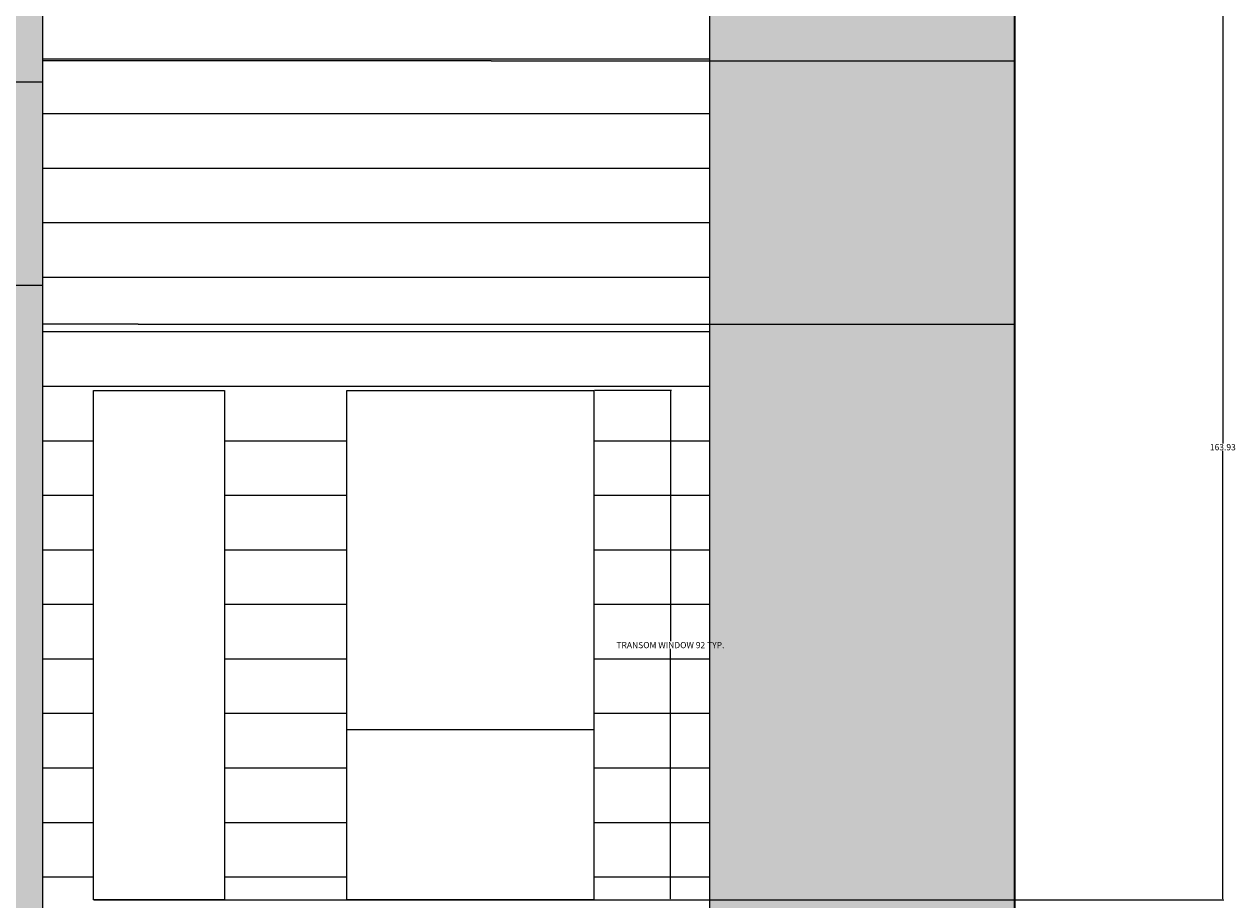
# Model space of a CAD drawing. Units: inches. Extents: x 8 to 634, y 41 to 867.
# Tile 9 of 21: x 415 to 634, y 124 to 283. Entities that reach past the tile are written whole.
import ezdxf

# ---------------------------------------------------------------- set-up
doc = ezdxf.new("R2010")
doc.units = ezdxf.units.IN
doc.header["$MEASUREMENT"] = 0
for name, color, linetype, lineweight in [('A-ANNO-DIMS', 2, 'Continuous', 18), ('A-GLAZ', 4, 'Continuous', 25), ('A-WALL', 7, 'Continuous', 35), ('A-WALL-PANL', 7, 'Continuous', 18), ('A-WALL-PATT', 8, 'Continuous', 9)]:
    doc.layers.add(name, color=color, linetype=linetype, lineweight=lineweight)
doc.styles.get("Standard").update_dxf_attribs({"font": 'arial.ttf'})
doc.dimstyles.get("Standard").update_dxf_attribs({"dimtxt": 1.125, "dimasz": 0.18, "dimexe": 0.18, "dimexo": 0.0625, "dimgap": 0.09, "dimtad": 0, "dimtih": 1, "dimtoh": 1, "dimdec": 4, "dimzin": 0, "dimdsep": 46, "dimlunit": 4, "dimtxsty": 'Standard', "dimcen": 0.09, "dimadec": 0, "dimazin": 0, "dimtfac": 1, "dimtdec": 4, "dimtofl": 0, "dimtmove": 0, "dimatfit": 3, "dimfxl": 1, "dimtolj": 1, "dimtzin": 0, "dimarcsym": 0})

# ---------------------------------------------------------------- blocks, each defined once
blk = doc.blocks.new('WIN-NARROW-FIXED')
blk.add_lwpolyline([(0, 92.26), (23.77, 92.26), (23.77, 0), (0, 0)], close=True)
blk = doc.blocks.new('WIN-WIDE-TRANSOM')
blk.add_line((0, 30.85), (44.78, 30.85))
blk.add_lwpolyline([(0, 92.26), (44.78, 92.26), (44.78, 0), (0, 0)], close=True)
blk = doc.blocks.new('*D9')
at = {"layer": 'A-ANNO-DIMS', "color": 0, "lineweight": -2, "transparency": 16777216}
for p, q in [((518.18, 216.5), (532.13, 216.5)), ((531.95, 216.32), (531.95, 171.04)), ((531.95, 124.41), (531.95, 169.69)), ((518.18, 124.23), (532.13, 124.23))]:
    blk.add_line(p, q, dxfattribs=at)
at = {"layer": 'A-ANNO-DIMS', "color": 0, "transparency": 16777216}
for points in [[(531.92, 216.32), (531.98, 216.32), (531.95, 216.5)], [(531.92, 124.41), (531.98, 124.41), (531.95, 124.23)]]:
    blk.add_solid(points, dxfattribs=at)
at = {"layer": 'Defpoints', "color": 0, "transparency": 16777216}
for p in [(518.11, 216.5), (531.95, 216.5), (518.11, 124.23)]:
    blk.add_point(p, dxfattribs=at)
at = {"layer": 'A-ANNO-DIMS', "color": 0, "transparency": 16777216, "insert": (531.95, 170.36), "char_height": 1.125, "attachment_point": 5}
blk.add_mtext('\\A1;TRANSOM WINDOW 92 TYP.', dxfattribs=at)
blk = doc.blocks.new('*D39')
at = {"layer": 'A-ANNO-DIMS', "color": 0, "lineweight": -2, "transparency": 16777216}
for p, q in [((427.5, 288.17), (632.18, 288.17)), ((632, 287.99), (632, 206.86)), ((632, 124.41), (632, 205.54)), ((427.5, 124.23), (632.18, 124.23))]:
    blk.add_line(p, q, dxfattribs=at)
at = {"layer": 'A-ANNO-DIMS', "color": 0, "transparency": 16777216}
for points in [[(631.97, 287.99), (632.03, 287.99), (632, 288.17)], [(631.97, 124.41), (632.03, 124.41), (632, 124.23)]]:
    blk.add_solid(points, dxfattribs=at)
at = {"layer": 'Defpoints', "color": 0, "transparency": 16777216}
for p in [(427.44, 288.17), (632, 288.17), (427.44, 124.23)]:
    blk.add_point(p, dxfattribs=at)
at = {"layer": 'A-ANNO-DIMS', "color": 0, "transparency": 16777216, "insert": (632, 206.2), "char_height": 1.125, "attachment_point": 5}
blk.add_mtext('\\A1;163.93', dxfattribs=at)

msp = doc.modelspace()

# ---------------------------------------------------------------- hatches: boundary and pattern name
at = {"layer": 'A-WALL-PATT', "transparency": 33554687}
h = msp.add_hatch(dxfattribs=at)
h.set_pattern_fill('ANSI31', color=256, scale=79, angle=135)
h.paths.add_polyline_path([(539.0002, 276.166), (499.4677, 276.166), (418.2881, 276.166), (418.2881, 228.4951), (435.5682, 228.4951), (539.0002, 228.4951)])
h.paths.add_polyline_path([(539.0002, 228.4951), (435.5682, 228.4951), (418.2881, 228.4951), (418.2881, 112.2342), (439.3242, 112.2342), (539.0002, 112.2342)])
h.paths.add_polyline_path([(518.1129, 124.2342), (473.3277, 124.2342), (473.3277, 216.4951), (518.1129, 216.4951)], flags=16)
h.paths.add_polyline_path([(451.2116, 124.2342), (427.4368, 124.2342), (427.4368, 216.4951), (451.2116, 216.4951)], flags=16)
h.paths.add_polyline_path([(539.0002, 112.2342), (439.3242, 112.2342), (418.2881, 112.2342), (418.2881, 91.5417), (539.0002, 91.5417)])
h.paths.add_polyline_path([(539.0002, 392.4268), (427.4368, 392.4268), (418.2881, 392.4268), (418.2881, 391.7598), (418.2881, 276.166), (499.4677, 276.166), (539.0002, 276.166)])
h.paths.add_polyline_path([(518.1129, 288.166), (473.3277, 288.166), (473.3277, 380.4268), (518.1129, 380.4268)], flags=16)
h.paths.add_polyline_path([(451.2116, 288.166), (427.4368, 288.166), (427.4368, 380.4268), (451.2116, 380.4268)], flags=16)
h.paths.add_polyline_path([(539.0002, 451.6305), (427.4368, 452.9097), (418.2881, 452.9097), (418.2881, 392.4268), (427.4368, 392.4268), (539.0002, 392.4268)])
h.paths.add_polyline_path([(539.0002, 569.1705), (427.4368, 569.1705), (418.2881, 569.1705), (418.2881, 452.9097), (427.4368, 452.9097), (539.0002, 451.6305)])
h.paths.add_polyline_path([(473.3277, 557.1705), (518.1129, 557.1705), (518.1129, 464.9097), (473.3277, 464.9097)], flags=16)
h.paths.add_polyline_path([(451.2116, 557.1705), (451.2116, 464.9097), (427.4368, 464.9097), (427.4368, 557.1705)], flags=16)
h.paths.add_polyline_path([(539.0002, 619.6298), (418.2881, 619.6298), (418.2881, 569.1705), (427.4368, 569.1705), (539.0002, 569.1705)])
h.paths.add_polyline_path([(556.7072, 774.3342), (556.7072, 776.8929), (299.7961, 776.8929), (299.7961, 697.6655), (322.56, 697.6655), (322.56, 740.5561), (355.7466, 740.5561), (355.7466, 697.6655), (360.785, 697.6655), (370.3877, 697.6655), (370.3877, 740.5561), (439.201, 740.5561), (439.201, 691.978), (449.4498, 691.978), (449.4498, 740.5561), (498.2535, 740.5561), (498.2535, 691.978), (508.5023, 691.978), (508.5023, 740.5561), (536.3204, 740.5561), (536.3204, 691.978), (539.0002, 691.978), (539.0002, 697.6655), (556.7072, 697.6655)])
h = msp.add_hatch(dxfattribs=at)
h.set_pattern_fill('AR-CONC', color=256, scale=3.2)
h.paths.add_polyline_path([(119.7065, 697.6655), (47.3401, 697.6655), (47.3401, 569.1705), (119.7065, 569.1705)])
h.paths.add_polyline_path([(202.1558, 697.6655), (119.7065, 697.6655), (119.7065, 569.1705), (202.1558, 569.1705)])
h.paths.add_polyline_path([(284.6051, 697.6655), (202.1558, 697.6655), (202.1558, 569.1705), (284.6051, 569.1705)])
h.paths.add_polyline_path([(119.7065, 569.1705), (47.3401, 569.1705), (47.3401, 523.5555), (47.3401, 449.7533), (119.7065, 449.7533)])
h.paths.add_polyline_path([(342.6544, 682.1444), (360.785, 697.6655), (284.6051, 697.6655), (284.6051, 569.1705), (342.6544, 569.1705)])
h.paths.add_polyline_path([(342.6544, 569.1705), (284.6051, 569.1705), (284.6051, 449.7533), (342.6544, 449.7533)])
h.paths.add_polyline_path([(418.2881, 691.978), (418.2881, 697.6655), (360.785, 697.6655), (360.785, 569.1705), (418.2881, 569.1705)])
h.paths.add_polyline_path([(418.2881, 569.1705), (360.785, 569.1705), (360.785, 523.5555), (360.785, 449.7533), (418.2881, 449.7533)])
h.paths.add_polyline_path([(594.3501, 697.6655), (539.0002, 697.6655), (539.0002, 691.978), (539.0002, 569.1705), (594.3501, 569.1705)])
h.paths.add_polyline_path([(594.3501, 523.5555), (594.3501, 569.1705), (539.0002, 569.1705), (539.0002, 451.6305), (594.3501, 451.6305)])
h.paths.add_polyline_path([(594.3501, 451.6305), (539.0002, 451.6305), (539.0002, 391.7598), (594.3501, 391.7598)])
h.paths.add_polyline_path([(594.3501, 391.7598), (539.0002, 391.7598), (539.0002, 276.166), (594.3501, 276.166)])
h.paths.add_polyline_path([(418.2881, 449.7533), (360.785, 449.7533), (360.785, 391.7598), (418.2881, 391.7598)])
h.paths.add_polyline_path([(342.6544, 449.7533), (284.6051, 449.7533), (284.6051, 391.7598), (342.6544, 391.7598)])
h.paths.add_polyline_path([(342.6544, 391.7598), (284.6051, 391.7598), (284.6051, 272.3426), (342.6544, 272.3426)])
h.paths.add_polyline_path([(418.2881, 391.7598), (360.785, 391.7598), (360.785, 272.3426), (418.2881, 272.3426)])
h.paths.add_polyline_path([(418.2881, 272.3426), (360.785, 272.3426), (360.785, 235.5555), (418.2881, 235.5555)])
h.paths.add_polyline_path([(342.6544, 272.3426), (284.6051, 272.3426), (284.6051, 235.5555), (295.0049, 235.5555), (342.6544, 235.5555)])
h.paths.add_polyline_path([(594.3501, 276.166), (539.0002, 276.166), (539.0002, 228.4951), (594.3501, 228.4951)])
h.paths.add_polyline_path([(594.3501, 228.4951), (539.0002, 228.4951), (539.0002, 91.5417), (594.3501, 91.5417)])
h.paths.add_polyline_path([(418.2881, 235.5555), (360.785, 235.5555), (360.785, 91.5417), (418.2881, 91.5417)])
h.paths.add_polyline_path([(284.6051, 272.3426), (119.7065, 272.3426), (119.7065, 235.5555), (284.6051, 235.5555)])
h.paths.add_polyline_path([(119.7065, 272.3426), (47.3401, 272.3426), (47.3401, 235.5555), (47.3401, 91.5555), (63.5448, 91.5555), (63.5448, 227.8036), (268.998, 227.8036), (268.998, 91.5555), (295.0049, 91.5555), (295.0049, 222.583), (271.9787, 222.583), (271.9787, 229.0481), (62.4019, 229.0481), (62.4019, 222.583), (61.1827, 222.583), (61.1827, 235.5555), (119.7065, 235.5555)])
h.paths.add_polyline_path([(119.7065, 391.7598), (47.3401, 391.7598), (47.3401, 379.5555), (47.3401, 272.3426), (119.7065, 272.3426)])
h.paths.add_polyline_path([(119.7065, 449.7533), (47.3401, 449.7533), (47.3401, 391.7598), (119.7065, 391.7598)])
h.paths.add_polyline_path([(202.1558, 449.7533), (119.7065, 449.7533), (119.7065, 391.7598), (202.1558, 391.7598)])
h.paths.add_polyline_path([(284.6051, 449.7533), (202.1558, 449.7533), (202.1558, 391.7598), (284.6051, 391.7598)])

# ---------------------------------------------------------------- linework, layer by layer
at = {"layer": 'A-WALL'}
msp.add_line((594.3501, 91.5417), (594.3501, 523.5555), dxfattribs=at)
at = {"layer": 'A-WALL-PANL'}
for p, q in [((499.4677, 276.166), (418.2881, 276.166)), ((499.4677, 276.166), (539.0002, 276.166)), ((539.0002, 276.166), (594.3501, 276.166)), ((284.6051, 272.3426), (418.2881, 272.3426)), ((360.785, 235.5555), (418.2881, 235.5555)), ((435.5682, 228.4951), (418.2881, 228.4951)), ((435.5682, 228.4951), (539.0002, 228.4951)), ((539.0002, 228.4951), (594.3501, 228.4951))]:
    msp.add_line(p, q, dxfattribs=at)
msp.add_lwpolyline([(539.0002, 691.978), (539.0002, 91.5417), (418.2881, 91.5417), (418.2881, 691.978)], dxfattribs=at)

# ---------------------------------------------------------------- block references
at = {"layer": 'A-GLAZ'}
for name, p in [('WIN-NARROW-FIXED', (427.437, 124.234)), ('WIN-WIDE-TRANSOM', (473.328, 124.234))]:
    msp.add_blockref(name, p, dxfattribs=at)

# ---------------------------------------------------------------- dimensions: what is measured, and where the dimension line sits
at = {"layer": 'A-ANNO-DIMS'}
dim = msp.add_linear_dim(base=(632.0001, 288.166), p1=(427.4368, 124.2342), p2=(427.4368, 288.166), angle=90, dimstyle='Standard', override={"dimdec": 2, "dimlfac": 1, "dimrnd": 0, "dimzin": 0, "dimdsep": 46, "dimlunit": 2}, dxfattribs=at)
dim.commit()
dim.dimension.update_dxf_attribs({"geometry": '*D39', "text_midpoint": (632.0001, 206.2001)})
dim = msp.add_linear_dim(base=(531.952, 216.4951), p1=(518.1129, 124.2342), p2=(518.1129, 216.4951), angle=90, text='TRANSOM WINDOW <> TYP.', dimstyle='Standard', override={"dimdec": 0, "dimlfac": 1, "dimrnd": 0, "dimzin": 0, "dimdsep": 46, "dimlunit": 2}, dxfattribs=at)
dim.commit()
dim.dimension.update_dxf_attribs({"geometry": '*D9', "text_midpoint": (531.952, 170.3647)})

doc.saveas('drawing.dxf')
